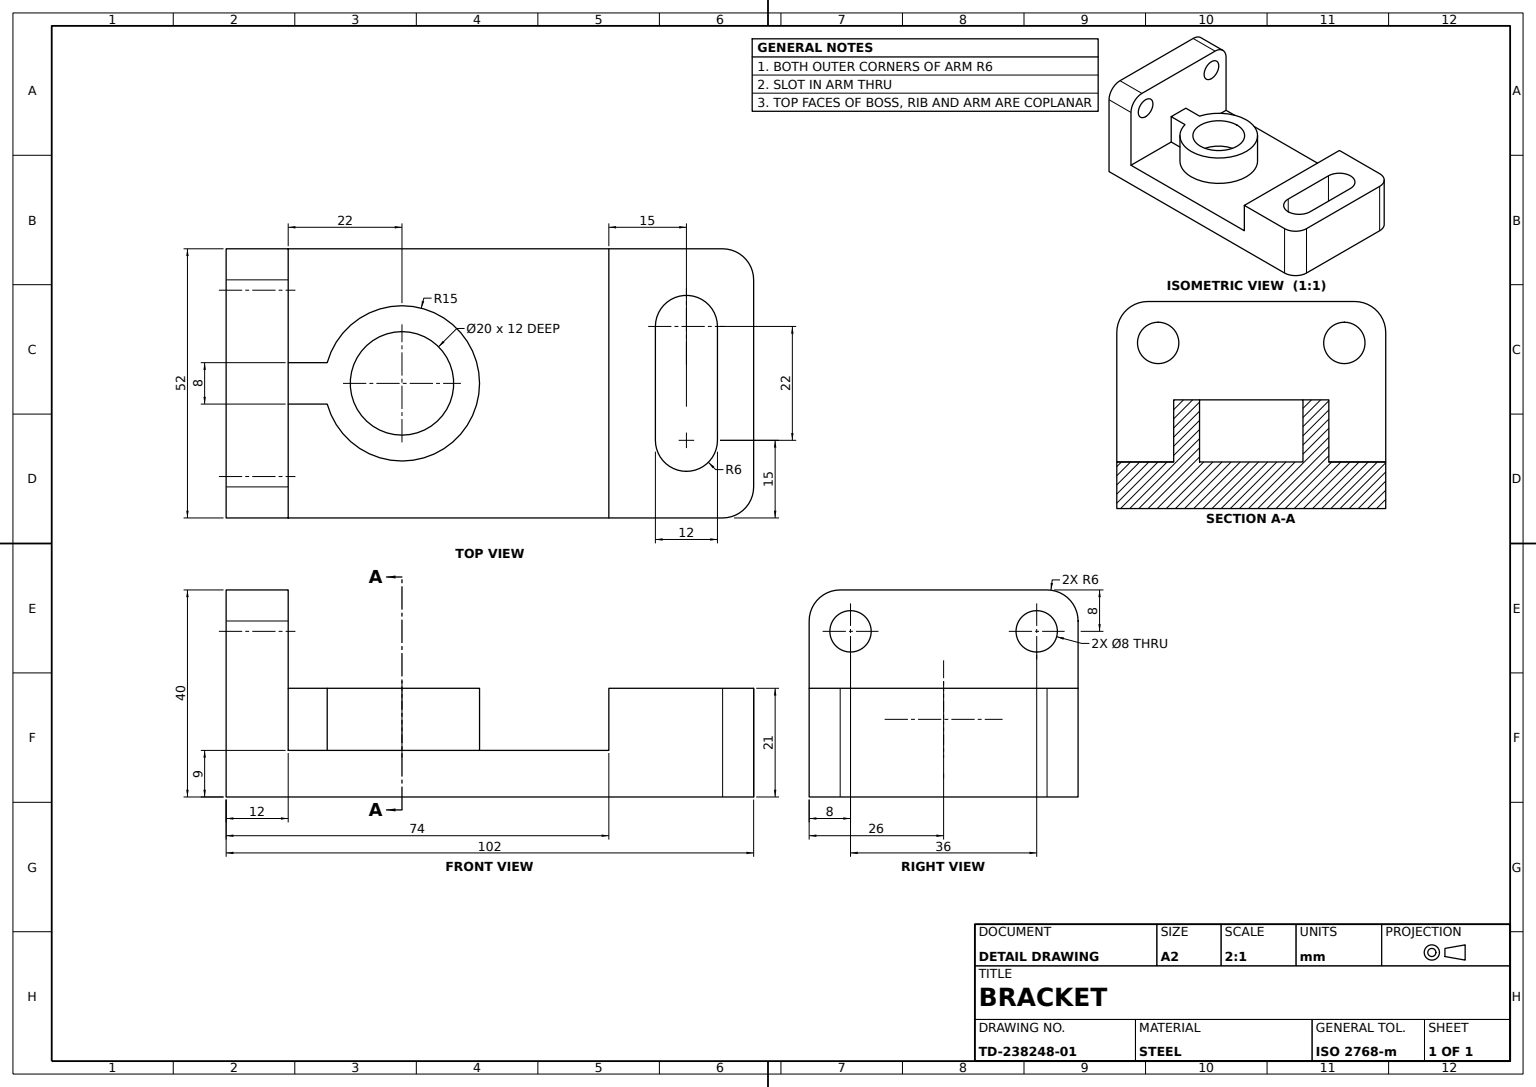
from build123d import *

# Parameters (mm, degrees)
BACK_PLATE_DEPTH          = 9
TOP_ARM_DEPTH             = 12
TOP_ARM_SLOT_DEPTH        = 21
BASE_FOOT_DEPTH           = 12
MOUNTING_HOLES_SKETCH_R   = 4
MOUNTING_HOLES_2X_8_DEPTH = 12
BEARING_BOSS_30_DEPTH     = 12
BORE_SKETCH_R             = 10
BORE_20_DEPTH             = 12


with BuildPart() as part:
    # Back Plate Sketch → Back Plate (new body)
    with BuildSketch(Plane.XY):
        with BuildLine():
            Line((0, 0), (52, 0))
            Line((52, 0), (52, 96))
            ThreePointArc((52, 96), (50.242640687, 100.242640687), (46, 102))
            Line((46, 102), (6, 102))
            ThreePointArc((6, 102), (1.757359313, 100.242640687), (0, 96))
            Line((0, 96), (0, 0))
        make_face()
    extrude(amount=BACK_PLATE_DEPTH)

    # Top Arm Sketch → Top Arm (add)
    with BuildSketch(Plane.XY.offset(9)):
        with BuildLine():
            Line((26, 74), (52, 74))
            Line((52, 74), (52, 96))
            ThreePointArc((52, 96), (50.242640687, 100.242640687), (46, 102))
            Line((46, 102), (6, 102))
            ThreePointArc((6, 102), (1.757359313, 100.242640687), (0, 96))
            Line((0, 96), (0, 74))
            Line((0, 74), (26, 74))
        make_face()
    extrude(amount=TOP_ARM_DEPTH)

    # Top Arm Slot Sketch → Top Arm Slot (cut)
    with BuildSketch(Plane.XY.offset(21)):
        with BuildLine():
            Line((26, 95), (15, 95))
            ThreePointArc((15, 95), (9, 89), (15, 83))
            Line((15, 83), (37, 83))
            ThreePointArc((37, 83), (43, 89), (37, 95))
            Line((37, 95), (26, 95))
        make_face()
    extrude(amount=-TOP_ARM_SLOT_DEPTH, mode=Mode.SUBTRACT)

    # Base Foot Sketch → Base Foot (add)
    with BuildSketch(Plane.XZ):
        with BuildLine():
            Line((0, 9), (0, 34))
            ThreePointArc((0, 34), (1.757359313, 38.242640687), (6, 40))
            Line((6, 40), (46, 40))
            ThreePointArc((46, 40), (50.242640687, 38.242640687), (52, 34))
            Line((52, 34), (52, 9))
            Line((52, 9), (52, 0))
            Line((52, 0), (0, 0))
            Line((0, 0), (0, 9))
        make_face()
    extrude(amount=-BASE_FOOT_DEPTH)

    # Mounting Holes Sketch → Mounting Holes 2xØ8 (cut)
    with BuildSketch(Plane(origin=(0, 12, 0), x_dir=(1, 0, 0), z_dir=(0, 1, 0))):
        with Locations(Location((8, -32, 0), (0, 0, 270))):
            Circle(MOUNTING_HOLES_SKETCH_R)
        with Locations(Location((44, -32, 0), (0, 0, 270))):
            Circle(MOUNTING_HOLES_SKETCH_R)
    extrude(amount=-MOUNTING_HOLES_2X_8_DEPTH, mode=Mode.SUBTRACT)

    # Bearing Boss Sketch → Bearing Boss Ø30 (add)
    with BuildSketch(Plane.XY.offset(9)):
        with BuildLine():
            Line((30, 19), (30, 12))
            Line((30, 12), (22, 12))
            Line((22, 12), (22, 19.543167705))
            ThreePointArc((22, 19.543167705), (26, 49), (30, 19.543167705))
            Line((30, 19.543167705), (30, 19))
        make_face()
    extrude(amount=BEARING_BOSS_30_DEPTH)

    # Bore Sketch → Bore Ø20 (cut)
    with BuildSketch(Plane.XY.offset(21)):
        with Locations((26, 34)):
            Circle(BORE_SKETCH_R)
    extrude(amount=-BORE_20_DEPTH, mode=Mode.SUBTRACT)


solid = part.part
